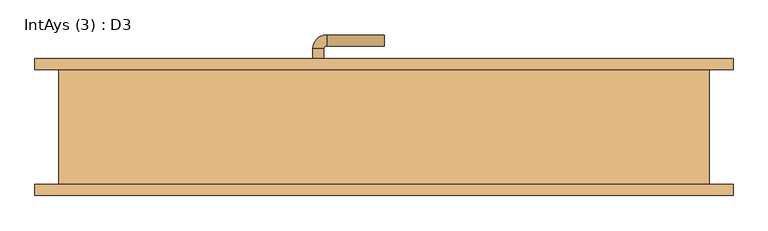
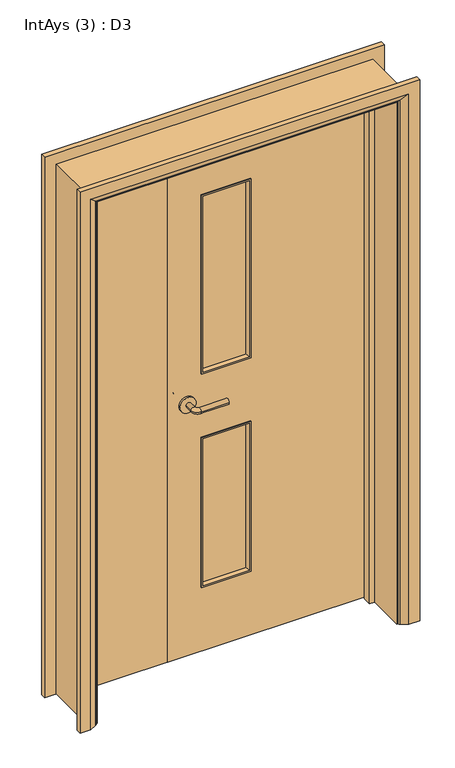
"""IFC4 building model written with IfcOpenShell, lengths in millimetres: door geometry, IntAys (3) : D3."""

from ifc_helpers import new_model, si_unit, point, frame, frame_2d, origin, place, context, project, spatial, polyline, circle_curve, ellipse_curve, trimmed, segment, composite_curve, outline, extrude, faceted_brep, source, transform, mapped, element, save
from ifc_brep_helpers import plane_surface, cylinder_surface, revolved_surface, advanced_brep


def intays_3_d3_2ab6a75b(model_context):
    return source(origin(), model_context, "Body", "SolidModel", [
        advanced_brep(
        [(109.5, 65.0, 1000.0), (129.5, 65.0, 1000.0), (129.5, 35.0, 1000.0), (109.5, 35.0, 1000.0), (134.5, 30.0, 1000.0), (134.5, 10.0, 1000.0), (239.5, 10.0, 1000.0), (239.5, 30.0, 1000.0)],
        [
            (0, 1, circle_curve(frame((119.5, 65.0, 1000.0), z_axis=(0.0, 1.0, 0.0), x_axis=(1.0, 0.0, 0.0)), 10.0)),
            (1, 0, circle_curve(frame((119.5, 65.0, 1000.0), z_axis=(0.0, 1.0, 0.0), x_axis=(1.0, 0.0, 0.0)), 10.0)),
            (1, 2),
            (2, 3, circle_curve(frame((119.5, 35.0, 1000.0), z_axis=(0.0, 1.0, 0.0), x_axis=(1.0, 0.0, 0.0)), 10.0)),
            (3, 0),
            (3, 2, circle_curve(frame((119.5, 35.0, 1000.0), z_axis=(0.0, 1.0, 0.0), x_axis=(1.0, 0.0, 0.0)), 10.0)),
            (4, 5, circle_curve(frame((134.5, 20.0, 1000.0), z_axis=(-1.0, 0.0, 0.0), x_axis=(0.0, 1.0, 0.0)), 10.0)),
            (5, 3, circle_curve(frame((134.5, 35.0, 1000.0), z_axis=(0.0, 0.0, -1.0), x_axis=(-1.0, 0.0, 0.0)), 25.0)),
            (2, 4, circle_curve(frame((134.5, 35.0, 1000.0), z_axis=(0.0, 0.0, 1.0), x_axis=(-1.0, 0.0, 0.0)), 5.0)),
            (5, 4, circle_curve(frame((134.5, 20.0, 1000.0), z_axis=(-1.0, 0.0, 0.0), x_axis=(0.0, 1.0, 0.0)), 10.0)),
            (6, 7, circle_curve(frame((239.5, 20.0, 1000.0), z_axis=(1.0, 0.0, 0.0), x_axis=(0.0, 1.0, 0.0)), 10.0)),
            (7, 6, circle_curve(frame((239.5, 20.0, 1000.0), z_axis=(1.0, 0.0, 0.0), x_axis=(0.0, 1.0, 0.0)), 10.0)),
            (4, 7),
            (6, 5),
        ],
        [
            plane_surface(frame((119.5, 65.0, 1000.0), z_axis=(0.0, 1.0, 0.0), x_axis=(0.0, 0.0, 1.0))),
            cylinder_surface(frame((119.5, 65.0, 1000.0), z_axis=(0.0, 1.0, 0.0), x_axis=(1.0, 0.0, 0.0)), 10.0),
            revolved_surface(trimmed(ellipse_curve(frame((119.5, 35.0, 1000.0), z_axis=(0.0, -1.0, 0.0), x_axis=(1.0, 0.0, 0.0)), 10.0, 10.0), [point((109.5, 35.0, 1000.0))], [point((129.5, 35.0, 1000.0))], True, "CARTESIAN"), (134.5, 35.0, 1000.0), (0.0, 0.0, -1.0)),
            revolved_surface(trimmed(ellipse_curve(frame((119.5, 35.0, 1000.0), z_axis=(0.0, -1.0, 0.0), x_axis=(1.0, 0.0, 0.0)), 10.0, 10.0), [point((129.5, 35.0, 1000.0))], [point((109.5, 35.0, 1000.0))], True, "CARTESIAN"), (134.5, 35.0, 1000.0), (0.0, 0.0, -1.0)),
            plane_surface(frame((239.5, 20.0, 1000.0), z_axis=(1.0, 0.0, 0.0), x_axis=(0.0, 0.0, 1.0))),
            cylinder_surface(frame((134.5, 20.0, 1000.0), z_axis=(-1.0, 0.0, 0.0), x_axis=(0.0, 1.0, 0.0)), 10.0),
        ],
        [
            (0, [[1, 2]]),
            (1, [[3, 4, 5, -2]]),
            (1, [[-5, 6, -3, -1]]),
            (2, [[7, 8, -4, 9]]),
            (3, [[10, -9, -6, -8]]),
            (4, [[11, 12]]),
            (5, [[13, -11, 14, -7]]),
            (5, [[-14, -12, -13, -10]]),
        ],
    ),
        extrude(outline(composite_curve([segment(trimmed(circle_curve(frame_2d((1000.0, 117.0)), 30.0), [point((1000.0, 87.0))], [point((1000.0, 147.0))], False, "CARTESIAN"), True, "CONTINUOUS"), segment(trimmed(circle_curve(frame_2d((1000.0, 117.0)), 30.0), [point((1000.0, 147.0))], [point((1000.0, 87.0))], False, "CARTESIAN"), True, "CONTINUOUS")], self_intersect=False)), frame((0.0, 65.0, 0.0), z_axis=(0.0, 1.0, 0.0), x_axis=(0.0, 0.0, 1.0)), (0.0, 0.0, 1.0), 8.0),
        advanced_brep(
        [(109.5, 113.0, 1000.0), (129.5, 113.0, 1000.0), (109.5, 143.0, 1000.0), (129.5, 143.0, 1000.0), (134.5, 148.0, 1000.0), (134.5, 168.0, 1000.0), (239.5, 168.0, 1000.0), (239.5, 148.0, 1000.0)],
        [
            (0, 1, circle_curve(frame((119.5, 113.0, 1000.0), z_axis=(0.0, -1.0, 0.0), x_axis=(1.0, 0.0, 0.0)), 10.0)),
            (1, 0, circle_curve(frame((119.5, 113.0, 1000.0), z_axis=(0.0, -1.0, 0.0), x_axis=(1.0, 0.0, 0.0)), 10.0)),
            (0, 2),
            (2, 3, circle_curve(frame((119.5, 143.0, 1000.0), z_axis=(0.0, -1.0, 0.0), x_axis=(1.0, 0.0, 0.0)), 10.0)),
            (3, 1),
            (3, 2, circle_curve(frame((119.5, 143.0, 1000.0), z_axis=(0.0, -1.0, 0.0), x_axis=(1.0, 0.0, 0.0)), 10.0)),
            (4, 3, circle_curve(frame((134.5, 143.0, 1000.0), z_axis=(0.0, 0.0, 1.0), x_axis=(-1.0, 0.0, 0.0)), 5.0)),
            (2, 5, circle_curve(frame((134.5, 143.0, 1000.0), z_axis=(0.0, 0.0, -1.0), x_axis=(-1.0, 0.0, 0.0)), 25.0)),
            (5, 4, circle_curve(frame((134.5, 158.0, 1000.0), z_axis=(-1.0, 0.0, 0.0), x_axis=(0.0, -1.0, 0.0)), 10.0)),
            (4, 5, circle_curve(frame((134.5, 158.0, 1000.0), z_axis=(-1.0, 0.0, 0.0), x_axis=(0.0, -1.0, 0.0)), 10.0)),
            (6, 7, circle_curve(frame((239.5, 158.0, 1000.0), z_axis=(1.0, 0.0, 0.0), x_axis=(0.0, -1.0, 0.0)), 10.0)),
            (7, 6, circle_curve(frame((239.5, 158.0, 1000.0), z_axis=(1.0, 0.0, 0.0), x_axis=(0.0, -1.0, 0.0)), 10.0)),
            (5, 6),
            (7, 4),
        ],
        [
            plane_surface(frame((119.5, 113.0, 1000.0), z_axis=(0.0, -1.0, 0.0), x_axis=(0.0, 0.0, 1.0))),
            cylinder_surface(frame((119.5, 113.0, 1000.0), z_axis=(0.0, -1.0, 0.0), x_axis=(1.0, 0.0, 0.0)), 10.0),
            revolved_surface(trimmed(ellipse_curve(frame((119.5, 143.0, 1000.0), z_axis=(0.0, -1.0, 0.0), x_axis=(1.0, 0.0, 0.0)), 10.0, 10.0), [point((109.5, 143.0, 1000.0))], [point((129.5, 143.0, 1000.0))], True, "CARTESIAN"), (134.5, 143.0, 1000.0), (0.0, 0.0, -1.0)),
            revolved_surface(trimmed(ellipse_curve(frame((119.5, 143.0, 1000.0), z_axis=(0.0, -1.0, 0.0), x_axis=(1.0, 0.0, 0.0)), 10.0, 10.0), [point((129.5, 143.0, 1000.0))], [point((109.5, 143.0, 1000.0))], True, "CARTESIAN"), (134.5, 143.0, 1000.0), (0.0, 0.0, -1.0)),
            plane_surface(frame((239.5, 158.0, 1000.0), z_axis=(1.0, 0.0, 0.0), x_axis=(0.0, 0.0, 1.0))),
            cylinder_surface(frame((134.5, 158.0, 1000.0), z_axis=(-1.0, 0.0, 0.0), x_axis=(0.0, -1.0, 0.0)), 10.0),
        ],
        [
            (0, [[1, 2]]),
            (1, [[-1, 3, 4, 5]]),
            (1, [[-2, -5, 6, -3]]),
            (2, [[7, -4, 8, 9]]),
            (3, [[-8, -6, -7, 10]]),
            (4, [[11, 12]]),
            (5, [[-9, 13, -12, 14]]),
            (5, [[-10, -14, -11, -13]]),
        ],
    ),
        extrude(outline(composite_curve([segment(trimmed(circle_curve(frame_2d((1000.0, 117.0)), 30.0), [point((1000.0, 87.0))], [point((1000.0, 147.0))], False, "CARTESIAN"), True, "CONTINUOUS"), segment(trimmed(circle_curve(frame_2d((1000.0, 117.0)), 30.0), [point((1000.0, 147.0))], [point((1000.0, 87.0))], False, "CARTESIAN"), True, "CONTINUOUS")], self_intersect=False)), frame((0.0, 105.0, 0.0), z_axis=(0.0, 1.0, 0.0), x_axis=(0.0, 0.0, 1.0)), (0.0, 0.0, 1.0), 8.0),
        extrude(outline(polyline([(2092.0, -353.0), (0.0, -353.0), (0.0, -321.0), (2060.0, -321.0), (2060.0, 799.0), (0.0, 799.0), (0.0, 831.0), (2092.0, 831.0), (2092.0, -353.0)])), frame((0.0, -105.0, 0.0), z_axis=(0.0, 1.0, 0.0), x_axis=(0.0, 0.0, 1.0)), (0.0, 0.0, 1.0), 210.0),
        faceted_brep([(-302.0, 70.0, 0.0), (-302.0, 38.0, 0.0), (-321.0, 38.0, 0.0), (-321.0, 70.0, 0.0), (-302.0, 70.0, 2041.0), (-302.0, 38.0, 2041.0), (-321.0, 38.0, 2060.0), (-321.0, 70.0, 2060.0), (780.0, 70.0, 0.0), (799.0, 70.0, 0.0), (799.0, 38.0, 0.0), (780.0, 38.0, 0.0), (780.0, 70.0, 2041.0), (799.0, 70.0, 2060.0), (799.0, 38.0, 2060.0), (780.0, 38.0, 2041.0)], [[[0, 1, 2, 3]], [[1, 0, 4, 5]], [[2, 1, 5, 6]], [[3, 2, 6, 7]], [[0, 3, 7, 4]], [[8, 9, 10, 11]], [[12, 13, 9, 8]], [[13, 14, 10, 9]], [[14, 15, 11, 10]], [[15, 12, 8, 11]], [[5, 4, 12, 15]], [[6, 5, 15, 14]], [[7, 6, 14, 13]], [[4, 7, 13, 12]]]),
        advanced_brep(
        [(874.0, 125.0, 0.0), (874.0, 105.0, 0.0), (804.0, 105.0, 0.0), (808.0, 111.0, 0.0), (834.0, 125.0, 0.0), (874.0, 125.0, 2135.0), (874.0, 105.0, 2135.0), (-396.0, 105.0, 2135.0), (-396.0, 105.0, 0.0), (-326.0, 105.0, 0.0), (-326.0, 105.0, 2065.0), (804.0, 105.0, 2065.0), (808.0, 111.0, 2069.0), (834.0, 125.0, 2095.0), (-356.0, 125.0, 2095.0), (-356.0, 125.0, 0.0), (-396.0, 125.0, 0.0), (-396.0, 125.0, 2135.0), (-330.0, 111.0, 0.0), (-330.0, 111.0, 2069.0)],
        [
            (0, 1),
            (1, 2),
            (2, 3, circle_curve(frame((812.0, 104.0, 0.0), z_axis=(0.0, 0.0, -1.0), x_axis=(1.0, 0.0, 0.0)), 8.0622577)),
            (3, 4),
            (4, 0),
            (0, 5),
            (5, 6),
            (6, 1),
            (6, 7),
            (7, 8),
            (8, 9),
            (9, 10),
            (10, 11),
            (11, 2),
            (11, 12, ellipse_curve(frame((812.0, 104.0, 2073.0), z_axis=(0.7071067811865475, 0.0, -0.7071067811865475), x_axis=(-0.7071067811865474, 0.0, -0.7071067811865476)), 11.4017543, 8.0622577)),
            (12, 3),
            (12, 13),
            (13, 4),
            (13, 14),
            (14, 15),
            (15, 16),
            (16, 17),
            (17, 5),
            (7, 17),
            (16, 8),
            (15, 18),
            (18, 9, circle_curve(frame((-334.0, 104.0, 0.0), z_axis=(0.0, 0.0, -1.0), x_axis=(-1.0, 0.0, 0.0)), 8.0622577)),
            (19, 10, ellipse_curve(frame((-334.0, 104.0, 2073.0), z_axis=(-0.7071067811865475, 0.0, -0.7071067811865475), x_axis=(-0.7071067811865474, 0.0, 0.7071067811865476)), 11.4017543, 8.0622577)),
            (18, 19),
            (14, 19),
            (19, 12),
        ],
        [
            plane_surface(frame((804.0, 105.0, 0.0), z_axis=(0.0, 0.0, -1.0), x_axis=(0.0, -1.0, 0.0))),
            plane_surface(frame((874.0, 125.0, 0.0), z_axis=(1.0, 0.0, 0.0), x_axis=(0.0, 0.0, 1.0))),
            plane_surface(frame((874.0, 105.0, 0.0), z_axis=(0.0, -1.0, 0.0), x_axis=(0.0, 0.0, 1.0))),
            cylinder_surface(frame((812.0, 104.0, 0.0), z_axis=(0.0, 0.0, -1.0), x_axis=(1.0, 0.0, 0.0)), 8.0622577),
            plane_surface(frame((808.0, 111.0, 0.0), z_axis=(-0.4740998230350126, 0.8804710999221779, 0.0), x_axis=(0.0, 0.0, 1.0))),
            plane_surface(frame((834.0, 125.0, 0.0), z_axis=(0.0, 1.0, 0.0), x_axis=(0.0, 0.0, 1.0))),
            plane_surface(frame((-396.0, 125.0, 2135.0), z_axis=(-1.0, 0.0, 0.0), x_axis=(0.0, 0.0, -1.0))),
            plane_surface(frame((-326.0, 105.0, 0.0), z_axis=(0.0, 0.0, -1.0), x_axis=(0.0, -1.0, 0.0))),
            cylinder_surface(frame((-334.0, 104.0, 2065.0), z_axis=(0.0, 0.0, 1.0), x_axis=(-1.0, 0.0, 0.0)), 8.0622577),
            plane_surface(frame((-330.0, 111.0, 2069.0), z_axis=(0.4740998230350183, 0.8804710999221749, 0.0), x_axis=(0.0, 0.0, -1.0))),
            plane_surface(frame((874.0, 125.0, 2135.0), z_axis=(0.0, 0.0, 1.0), x_axis=(-1.0, 0.0, 0.0))),
            cylinder_surface(frame((804.0, 104.0, 2073.0), z_axis=(1.0, 0.0, 0.0), x_axis=(0.0, 0.0, 1.0)), 8.0622577),
            plane_surface(frame((808.0, 111.0, 2069.0), z_axis=(0.0, 0.8804710999221763, -0.4740998230350154), x_axis=(-1.0, 0.0, 0.0))),
        ],
        [
            (0, [[1, 2, 3, 4, 5]]),
            (1, [[-1, 6, 7, 8]]),
            (2, [[-2, -8, 9, 10, 11, 12, 13, 14]]),
            (3, [[-3, -14, 15, 16]]),
            (4, [[-4, -16, 17, 18]]),
            (5, [[-5, -18, 19, 20, 21, 22, 23, -6]]),
            (6, [[24, -22, 25, -10]]),
            (7, [[-21, 26, 27, -11, -25]]),
            (8, [[28, -12, -27, 29]]),
            (9, [[30, -29, -26, -20]]),
            (10, [[-7, -23, -24, -9]]),
            (11, [[-15, -13, -28, 31]]),
            (12, [[-17, -31, -30, -19]]),
        ],
    ),
        advanced_brep(
        [(-396.0, -125.0, 0.0), (-396.0, -105.0, 0.0), (-326.0, -105.0, 0.0), (-330.0, -111.0, 0.0), (-356.0, -125.0, 0.0), (-396.0, -125.0, 2135.0), (-396.0, -105.0, 2135.0), (874.0, -105.0, 2135.0), (874.0, -105.0, 0.0), (804.0, -105.0, 0.0), (804.0, -105.0, 2065.0), (-326.0, -105.0, 2065.0), (-330.0, -111.0, 2069.0), (-356.0, -125.0, 2095.0), (834.0, -125.0, 2095.0), (834.0, -125.0, 0.0), (874.0, -125.0, 0.0), (874.0, -125.0, 2135.0), (808.0, -111.0, 0.0), (808.0, -111.0, 2069.0)],
        [
            (0, 1),
            (1, 2),
            (2, 3, circle_curve(frame((-334.0, -104.0, 0.0), z_axis=(0.0, 0.0, -1.0), x_axis=(-1.0, 0.0, 0.0)), 8.0622577)),
            (3, 4),
            (4, 0),
            (0, 5),
            (5, 6),
            (6, 1),
            (6, 7),
            (7, 8),
            (8, 9),
            (9, 10),
            (10, 11),
            (11, 2),
            (11, 12, ellipse_curve(frame((-334.0, -104.0, 2073.0), z_axis=(-0.7071067811865475, 0.0, -0.7071067811865475), x_axis=(0.7071067811865474, 0.0, -0.7071067811865476)), 11.4017543, 8.0622577)),
            (12, 3),
            (12, 13),
            (13, 4),
            (13, 14),
            (14, 15),
            (15, 16),
            (16, 17),
            (17, 5),
            (7, 17),
            (16, 8),
            (15, 18),
            (18, 9, circle_curve(frame((812.0, -104.0, 0.0), z_axis=(0.0, 0.0, -1.0), x_axis=(1.0, 0.0, 0.0)), 8.0622577)),
            (19, 10, ellipse_curve(frame((812.0, -104.0, 2073.0), z_axis=(0.7071067811865475, 0.0, -0.7071067811865475), x_axis=(0.7071067811865474, 0.0, 0.7071067811865476)), 11.4017543, 8.0622577)),
            (18, 19),
            (14, 19),
            (19, 12),
        ],
        [
            plane_surface(frame((-326.0, -105.0, 0.0), z_axis=(0.0, 0.0, -1.0), x_axis=(0.0, -1.0, 0.0))),
            plane_surface(frame((-396.0, -125.0, 0.0), z_axis=(-1.0, 0.0, 0.0), x_axis=(0.0, 0.0, 1.0))),
            plane_surface(frame((-396.0, -105.0, 0.0), z_axis=(0.0, 1.0, 0.0), x_axis=(0.0, 0.0, 1.0))),
            cylinder_surface(frame((-334.0, -104.0, 0.0), z_axis=(0.0, 0.0, -1.0), x_axis=(-1.0, 0.0, 0.0)), 8.0622577),
            plane_surface(frame((-330.0, -111.0, 0.0), z_axis=(0.4740998230350183, -0.8804710999221749, 0.0), x_axis=(0.0, 0.0, 1.0))),
            plane_surface(frame((-356.0, -125.0, 0.0), z_axis=(0.0, -1.0, 0.0), x_axis=(0.0, 0.0, 1.0))),
            plane_surface(frame((874.0, -125.0, 2135.0), z_axis=(1.0, 0.0, 0.0), x_axis=(0.0, 0.0, -1.0))),
            plane_surface(frame((804.0, -105.0, 0.0), z_axis=(0.0, 0.0, -1.0), x_axis=(0.0, -1.0, 0.0))),
            cylinder_surface(frame((812.0, -104.0, 2065.0), z_axis=(0.0, 0.0, 1.0), x_axis=(1.0, 0.0, 0.0)), 8.0622577),
            plane_surface(frame((808.0, -111.0, 2069.0), z_axis=(-0.4740998230350183, -0.8804710999221749, 0.0), x_axis=(0.0, 0.0, -1.0))),
            plane_surface(frame((-396.0, -125.0, 2135.0), z_axis=(0.0, 0.0, 1.0), x_axis=(1.0, 0.0, 0.0))),
            cylinder_surface(frame((-326.0, -104.0, 2073.0), z_axis=(-1.0, 0.0, 0.0), x_axis=(0.0, 0.0, 1.0)), 8.0622577),
            plane_surface(frame((-330.0, -111.0, 2069.0), z_axis=(0.0, -0.8804710999221749, -0.4740998230350183), x_axis=(1.0, 0.0, 0.0))),
        ],
        [
            (0, [[1, 2, 3, 4, 5]]),
            (1, [[-1, 6, 7, 8]]),
            (2, [[-2, -8, 9, 10, 11, 12, 13, 14]]),
            (3, [[-3, -14, 15, 16]]),
            (4, [[-4, -16, 17, 18]]),
            (5, [[-5, -18, 19, 20, 21, 22, 23, -6]]),
            (6, [[24, -22, 25, -10]]),
            (7, [[-21, 26, 27, -11, -25]]),
            (8, [[28, -12, -27, 29]]),
            (9, [[30, -29, -26, -20]]),
            (10, [[-7, -23, -24, -9]]),
            (11, [[-15, -13, -28, 31]]),
            (12, [[-17, -31, -30, -19]]),
        ],
    ),
        extrude(outline(polyline([(5.753223, 796.0), (2057.0, 796.0), (2057.0, 46.0), (5.753223, 46.0), (5.753223, 796.0)]), holes=[polyline([(1807.0, 171.0), (1807.0, 356.0), (1100.0, 356.0), (1100.0, 171.0), (1807.0, 171.0)]), polyline([(850.0, 356.0), (257.0, 356.0), (257.0, 171.0), (850.0, 171.0), (850.0, 356.0)])]), frame((0.0, 73.0, 0.0), z_axis=(0.0, 1.0, 0.0), x_axis=(0.0, 0.0, 1.0)), (0.0, 0.0, 1.0), 32.0),
        extrude(outline(polyline([(43.0, 73.0), (-318.0, 73.0), (-318.0, 105.0), (43.0, 105.0), (43.0, 73.0)])), frame((0.0, 0.0, 5.753223), z_axis=(0.0, 0.0, 1.0), x_axis=(1.0, 0.0, 0.0)), (0.0, 0.0, 1.0), 2051.246777),
        extrude(outline(polyline([(356.0, 83.0), (171.0, 83.0), (171.0, 95.0), (356.0, 95.0), (356.0, 83.0)])), frame((0.0, 0.0, 1100.0), z_axis=(0.0, 0.0, 1.0), x_axis=(1.0, 0.0, 0.0)), (0.0, 0.0, 1.0), 707.0),
        extrude(outline(polyline([(356.0, 83.0), (171.0, 83.0), (171.0, 95.0), (356.0, 95.0), (356.0, 83.0)])), frame((0.0, 0.0, 257.0), z_axis=(0.0, 0.0, 1.0), x_axis=(1.0, 0.0, 0.0)), (0.0, 0.0, 1.0), 593.0),
        faceted_brep([(171.0, 108.0, 1100.0), (171.0, 95.0, 1100.0), (171.0, 95.0, 1807.0), (171.0, 108.0, 1807.0), (183.0, 95.0, 1112.0), (177.0, 108.0, 1106.0), (177.0, 108.0, 1801.0), (183.0, 95.0, 1795.0), (356.0, 95.0, 1807.0), (356.0, 108.0, 1807.0), (350.0, 108.0, 1801.0), (344.0, 95.0, 1795.0), (356.0, 95.0, 1100.0), (356.0, 108.0, 1100.0), (350.0, 108.0, 1106.0), (344.0, 95.0, 1112.0)], [[[0, 1, 2, 3]], [[4, 5, 6, 7]], [[3, 2, 8, 9]], [[7, 6, 10, 11]], [[9, 8, 12, 13]], [[11, 10, 14, 15]], [[1, 12, 8, 2], [7, 11, 15, 4]], [[13, 12, 1, 0]], [[3, 9, 13, 0], [5, 14, 10, 6]], [[15, 14, 5, 4]]]),
        faceted_brep([(356.0, 70.0, 1100.0), (356.0, 83.0, 1100.0), (356.0, 83.0, 1807.0), (356.0, 70.0, 1807.0), (344.0, 83.0, 1112.0), (350.0, 70.0, 1106.0), (350.0, 70.0, 1801.0), (344.0, 83.0, 1795.0), (171.0, 83.0, 1807.0), (171.0, 70.0, 1807.0), (177.0, 70.0, 1801.0), (183.0, 83.0, 1795.0), (171.0, 83.0, 1100.0), (171.0, 70.0, 1100.0), (177.0, 70.0, 1106.0), (183.0, 83.0, 1112.0)], [[[0, 1, 2, 3]], [[4, 5, 6, 7]], [[3, 2, 8, 9]], [[7, 6, 10, 11]], [[9, 8, 12, 13]], [[11, 10, 14, 15]], [[1, 12, 8, 2], [7, 11, 15, 4]], [[13, 12, 1, 0]], [[3, 9, 13, 0], [5, 14, 10, 6]], [[15, 14, 5, 4]]]),
        faceted_brep([(356.0, 70.0, 257.0), (356.0, 83.0, 257.0), (356.0, 83.0, 850.0), (356.0, 70.0, 850.0), (344.0, 83.0, 269.0), (350.0, 70.0, 263.0), (350.0, 70.0, 844.0), (344.0, 83.0, 838.0), (171.0, 83.0, 850.0), (171.0, 70.0, 850.0), (177.0, 70.0, 844.0), (183.0, 83.0, 838.0), (171.0, 83.0, 257.0), (171.0, 70.0, 257.0), (177.0, 70.0, 263.0), (183.0, 83.0, 269.0)], [[[0, 1, 2, 3]], [[4, 5, 6, 7]], [[3, 2, 8, 9]], [[7, 6, 10, 11]], [[9, 8, 12, 13]], [[11, 10, 14, 15]], [[1, 12, 8, 2], [7, 11, 15, 4]], [[13, 12, 1, 0]], [[3, 9, 13, 0], [5, 14, 10, 6]], [[15, 14, 5, 4]]]),
        faceted_brep([(171.0, 108.0, 257.0), (171.0, 95.0, 257.0), (171.0, 95.0, 850.0), (171.0, 108.0, 850.0), (183.0, 95.0, 269.0), (177.0, 108.0, 263.0), (177.0, 108.0, 844.0), (183.0, 95.0, 838.0), (356.0, 95.0, 850.0), (356.0, 108.0, 850.0), (350.0, 108.0, 844.0), (344.0, 95.0, 838.0), (356.0, 95.0, 257.0), (356.0, 108.0, 257.0), (350.0, 108.0, 263.0), (344.0, 95.0, 269.0)], [[[0, 1, 2, 3]], [[4, 5, 6, 7]], [[3, 2, 8, 9]], [[7, 6, 10, 11]], [[9, 8, 12, 13]], [[11, 10, 14, 15]], [[1, 12, 8, 2], [7, 11, 15, 4]], [[13, 12, 1, 0]], [[3, 9, 13, 0], [5, 14, 10, 6]], [[15, 14, 5, 4]]]),
    ])


if __name__ == "__main__":
    model = new_model("IFC4")
    model_context = context("Model", 3, world=origin())
    ifc_project = project(units=[si_unit("LENGTHUNIT", "METRE", prefix="MILLI")], contexts=[model_context])
    site = spatial("IfcSite", under=ifc_project)
    building = spatial("IfcBuilding", under=site)
    placement = place(None, origin())
    intays_3_d3_shape = intays_3_d3_2ab6a75b(model_context)
    element("IfcDoor", 1, ObjectType="IntAys (3) : D3", at=placement, inside=building, context=model_context, shape_type="MappedRepresentation", body=[
        mapped(intays_3_d3_shape, transform((0.0, 0.0, 0.0), x_axis=(1.0, 0.0, 0.0), y_axis=(0.0, 1.0, 0.0), z_axis=(0.0, 0.0, 1.0))),
    ])
    save(model, "model.ifc")

# Revit data of these elements
# Type "IntAys (3) : D3"
#   Type Mark = "57"
#   Type Comments = "Internal Asymmetric"
#   Operation = "DoubleDoorSingleSwing"
#   Keynote = "L20"
#   Description = "Internal Asymmetric Door"
#   VisionPanel Width = 185 mm
#   Thickness = 32 mm
#   Stop Thickness = 19 mm
#   Stop Depth = 32 mm
#   Stile Top of Lock Rail = 1100 mm
#   Stile Top Rail = 250 mm
#   Stile Shutting = 125 mm
#   Stile Lock Rail = 250 mm
#   Stile Intermediate/Frieze = 100 mm
#   Stile Bottom Rail = 250 mm
#   Secondary Panel Width = 361 mm
#   Rough Width = 1200 mm
#   Rough Height = 2100 mm
#   Main Panel Width = 750 mm
#   Handle Z Distance = 1000 mm
#   Handle X Distance = 75 mm
#   Handle Length = 350 mm
#   Frame Thickness = 32 mm
#   Door Panel Width = 750 mm
#   Door Panel Thickness = 32 mm
#   Height = 2100 mm
#   Door Panel Offset = 0 mm
#   Structural Tolerance = 8 mm
#   Tolerance = 3 mm
#   UnderCut = 7 mm
#   Width = 1200 mm
#   Door Panel Height = 2050 mm
#   Architrave Setback = 5 mm
#   Vis - Swing Single = yes
#   Vis - Swing Opposing = no
#   Vis - Swing Double = no
#   Vis - Stops = yes
#   Vis - Ironmongery = yes
#   Material Ironmongery = Door - Handle
#   Material Glass = Door - Glazing
#   Material Frame = Door - Frame/Mullion
#   Material Door = Door - Panel
#   Material Beading = Door - Panel
#   Material Architrave = Door - Architrave
#   Handle Style = element 420585
#   Function = (empty or 0)
#   Wall Closure = (empty or 0)
# Element 1 (IfcDoor, "IntAys (3) : D3")
#   Materials on its faces: "Door - Panel", "Door - Architrave", "Door - Handle", "Door - Frame/Mullion", "Door - Glazing"
# Materials
#   "Door - Handle": colour RGB 0 0 0, transparency 0, Keynote = "P21", Cost = 0, Export to IFC = 0
#   "Door - Glazing": colour RGB 0 0 255, transparency 0.75
#   "Door - Frame/Mullion": class "Wood", colour RGB 212 179 113, transparency 0, Keynote = "L20", Cost = 0, Export to IFC = 0
#   "Door - Panel": class "Wood", colour RGB 210 159 95, transparency 0, Keynote = "L20", Cost = 0, Export to IFC = 0
#   "Door - Architrave": class "Wood", colour RGB 154 90 5, transparency 0, Keynote = "P20", Cost = 0, Export to IFC = 0
